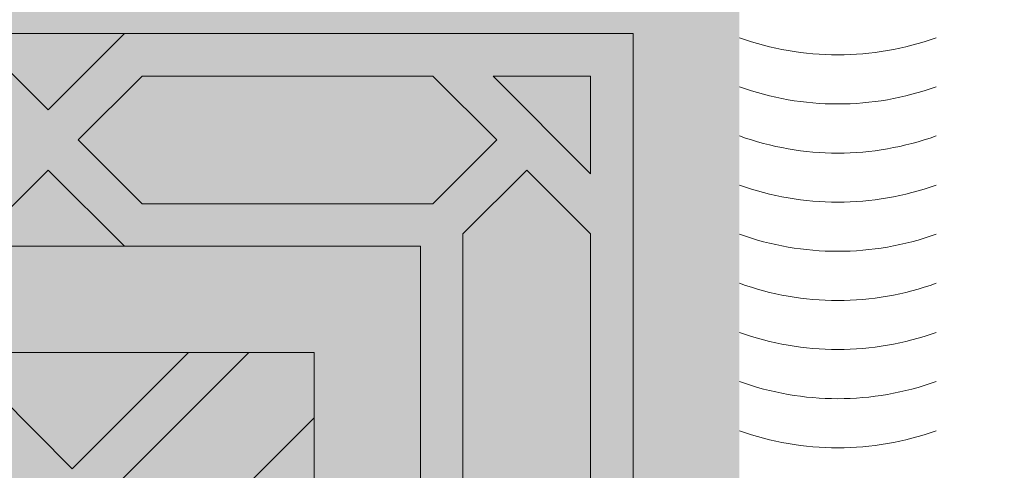
# Model space of a CAD drawing. Units: inches. Extents: x 844 to 2234, y 346 to 1084.
# Tile 86 of 93: x 2006.557 to 2012.46, y 710.224 to 712.926. Entities that reach past the tile are written whole.
import ezdxf

# ---------------------------------------------------------------- set-up
doc = ezdxf.new("R2010")
doc.units = ezdxf.units.IN
doc.header["$MEASUREMENT"] = 0
for name, color, linetype, lineweight in [('A-ANNO-DIMS', 2, 'Continuous', 18), ('furniture', 8, 'Continuous', 18), ('RA-AP-01$0$INT', 35, 'Continuous', 5)]:
    doc.layers.add(name, color=color, linetype=linetype, lineweight=lineweight)
doc.layers.add('RA-AP-01$0$FURN', color=3, linetype='Continuous')
doc.styles.get("Standard").update_dxf_attribs({"font": 'arial.ttf'})
doc.dimstyles.get("Standard").update_dxf_attribs({"dimtxt": 6, "dimasz": 3, "dimexe": 0.18, "dimexo": 0.0625, "dimgap": 0.09, "dimtad": 0, "dimtih": 1, "dimtoh": 1, "dimdec": 1, "dimzin": 0, "dimdsep": 46, "dimlunit": 3, "dimtxsty": 'Standard', "dimblk": 'ARCHTICK', "dimcen": 0.09, "dimadec": 0, "dimazin": 0, "dimtfac": 1, "dimtdec": 1, "dimtofl": 0, "dimtmove": 0, "dimatfit": 3, "dimfxl": 1, "dimtolj": 1, "dimtzin": 0, "dimarcsym": 0})

# ---------------------------------------------------------------- blocks, each defined once
blk = doc.blocks.new('A$C18D01794')
at = {"layer": 'RA-AP-01$0$INT'}
h = blk.add_hatch(color=256, dxfattribs=at)
h.paths.add_polyline_path([(4.355206456958071, -6.156712009588037), (4.355206456958071, -8.056712009588038), (5.455206456958072, -8.056712009588038), (5.455206456958072, -6.156712009588037)])
h.paths.add_polyline_path([(4.405206456958072, -8.006712009588039), (4.405206456958072, -6.206712009588038), (5.405206456958072, -6.206712009588038), (5.405206456958072, -8.006712009588039)], flags=16)
h = blk.add_hatch(color=256, dxfattribs=at)
h.paths.add_polyline_path([(4.505206456958071, -7.585498806127123), (4.46934859260189, -7.549640941759413), (4.505206456958071, -7.513783077414768), (4.505206456958071, -7.381963272220687), (4.469348592616735, -7.346105407867824), (4.505206456958071, -7.310247543514964), (4.505206456958071, -7.178427738324996), (4.469348592586679, -7.142569873965138), (4.505206456952245, -7.106712009588038), (4.476922185709333, -7.106712009588038), (4.455206456960671, -7.128427738343681), (4.433490728198047, -7.106712009588038), (4.405206456946033, -7.106712009588036), (4.441064321339216, -7.142569873969684), (4.40520645695807, -7.178427738362358), (4.405206456958072, -7.310247543472698), (4.441064321364728, -7.346105407867826), (4.40520645695807, -7.381963272262947), (4.40520645695807, -7.513783077378263), (4.441064321354429, -7.549640941786153), (4.405206456958072, -7.585498806170974), (4.405206456958072, -7.717318611286652), (4.441064321333084, -7.753176475673194), (4.405206456958072, -7.789034340036673), (4.405206456958072, -8.006712009588039), (4.644348592588106, -8.006712009588039), (4.680206456964639, -7.970854145211967), (4.716064321341165, -8.006712009588039), (4.869348592586113, -8.006712009588039), (4.905206456964143, -7.970854145210465), (4.941064321342174, -8.006712009588039), (5.094348592587118, -8.006712009588037), (5.130206456963649, -7.970854145211967), (5.166064321340178, -8.006712009588039), (5.405206456958072, -8.006712009588039), (5.405206456958072, -7.789034340024526), (5.369348592595202, -7.753176475673196), (5.40520645695807, -7.717318611298797), (5.40520645695807, -7.585498806158829), (5.369348592573859, -7.549640941786151), (5.40520645695807, -7.51378307739041), (5.40520645695807, -7.381963272250803), (5.36934859256356, -7.346105407867824), (5.405206456958072, -7.310247543484846), (5.405206456958072, -7.178427738350217), (5.369348592589068, -7.142569873969682), (5.405206456982249, -7.106712009588038), (5.376922185730244, -7.106712009588038), (5.355206456967613, -7.128427738343679), (5.333490728218955, -7.10671200958804), (5.305206456976043, -7.106712009588042), (5.341064321341609, -7.142569873965136), (5.305206456958072, -7.178427738337141), (5.305206456958072, -7.310247543502816), (5.34106432131155, -7.346105407867824), (5.305206456958072, -7.381963272232832), (5.30520645695807, -7.513783077402624), (5.341064321326395, -7.549640941759413), (5.305206456958072, -7.585498806139263), (5.305206456958072, -7.717318611299605), (5.341064321347738, -7.753176475677737), (5.305206456958072, -7.78903434007894), (5.30520645695807, -7.906712009588039), (5.166064321336834, -7.906712009588039), (5.130206456963647, -7.942569873961684), (5.094348592590464, -7.906712009588039), (4.941064321338827, -7.906712009588041), (4.905206456964145, -7.942569873963183), (4.869348592589459, -7.906712009588039), (4.716064321337822, -7.906712009588041), (4.680206456964641, -7.942569873961684), (4.644348592591453, -7.906712009588039), (4.505206456958071, -7.906712009588039), (4.505206456958071, -7.789034340066795), (4.469348592580545, -7.753176475677738), (4.505206456958071, -7.717318611311748)])
h.paths.add_polyline_path([(4.485206456974132, -7.709034340046354), (4.45520645695909, -7.739034340051736), (4.425206456974128, -7.709034340057131), (4.425206456993394, -7.593783077384998), (4.45520645699153, -7.563783077396511), (4.485206456993396, -7.593783077408017)], flags=16)
h.paths.add_polyline_path([(4.455206456954537, -7.767318611299197), (4.485206456958242, -7.797318611312542), (4.48520645695951, -7.912569873958716), (4.45520645695415, -7.942569873954422), (4.425206456957888, -7.912569873967813), (4.425206456957888, -7.797318611286197)], flags=16)
h.paths.add_polyline_path([(4.455206456964794, -7.535498806149051), (4.42520645696469, -7.5054988061393), (4.425206456983954, -7.390247543486406), (4.455206456990734, -7.360247543489279), (4.485206456983953, -7.39024754349214), (4.485206456964687, -7.505498806158811)], flags=16)
h.paths.add_polyline_path([(4.499348592588947, -7.926712009585049), (4.636064321340932, -7.926712009585049), (4.666064321342317, -7.956712009586821), (4.636064321343707, -7.986712009585048), (4.499348592575121, -7.986712009585048), (4.469348592591685, -7.956712009591957)], flags=16)
h.paths.add_polyline_path([(4.425206456957888, -7.940854145195974), (4.471064321332215, -7.986712009585049), (4.425206456957888, -7.986712009585049)], flags=16)
h.paths.add_polyline_path([(4.455206456990734, -7.331963272246367), (4.425206456989053, -7.301963272254337), (4.425206456969784, -7.186712009596224), (4.455206456965226, -7.156712009591144), (4.485206456969787, -7.186712009586051), (4.485206456989053, -7.301963272238404)], flags=16)
h.paths.add_polyline_path([(4.72434859258714, -7.926712009586255), (4.861064321340141, -7.926712009586248), (4.891064321340324, -7.956712009586823), (4.861064321340513, -7.986712009586252), (4.724348592586768, -7.986712009586252), (4.694348592586956, -7.956712009586821)], flags=16)
h.paths.add_polyline_path([(4.919348592587961, -7.956712009586821), (4.949348592588145, -7.92671200958625), (5.08606432134115, -7.926712009586253), (5.116064321341327, -7.956712009586823), (5.086064321341519, -7.986712009586252), (4.949348592587774, -7.986712009586252)], flags=16)
h.paths.add_polyline_path([(5.144348592585967, -7.956712009586823), (5.174348592587358, -7.926712009585049), (5.311064321339338, -7.926712009585049), (5.3410643213366, -7.956712009591957), (5.311064321353163, -7.986712009585048), (5.174348592584576, -7.986712009585048)], flags=16)
h.paths.add_polyline_path([(5.32520645693489, -7.593783077408021), (5.355206456936755, -7.563783077396511), (5.385206456934894, -7.593783077384998), (5.38520645695416, -7.709034340057128), (5.355206456969194, -7.739034340051736), (5.325206456954153, -7.709034340046352)], flags=16)
h.paths.add_polyline_path([(5.325206456970042, -7.797318611312542), (5.355206456973747, -7.767318611299197), (5.385206456970398, -7.7973186112862), (5.385206456970398, -7.912569873967816), (5.355206456974136, -7.942569873954422), (5.325206456968778, -7.912569873958716)], flags=16)
h.paths.add_polyline_path([(5.325206456963599, -7.505498806158811), (5.325206456944333, -7.39024754349214), (5.355206456937552, -7.360247543489279), (5.385206456944332, -7.39024754348641), (5.385206456963596, -7.505498806139303), (5.355206456963492, -7.53549880614905)], flags=16)
h.paths.add_polyline_path([(5.32520645693923, -7.301963272238403), (5.3252064569585, -7.186712009586051), (5.355206456963062, -7.156712009591142), (5.3852064569585, -7.186712009596224), (5.385206456939234, -7.301963272254338), (5.355206456937552, -7.331963272246369)], flags=16)
h.paths.add_polyline_path([(5.339348592596071, -7.986712009585048), (5.385206456970398, -7.940854145195972), (5.385206456970396, -7.986712009585048)], flags=16)
h = blk.add_hatch(color=256, dxfattribs=at)
h.paths.add_polyline_path([(4.469348592586677, -7.142569873965136), (4.505206456958073, -7.178427738324996), (4.505206456958071, -7.106712009582215)])
h.paths.add_polyline_path([(4.455206456960671, -7.128427738343681), (4.476922185709333, -7.106712009588038), (4.433490728198045, -7.106712009588038)])
h.paths.add_polyline_path([(4.405206456958073, -7.178427738362358), (4.441064321339218, -7.142569873969684), (4.40520645695807, -7.106712009600073)])
h.paths.add_polyline_path([(4.425206456989053, -7.301963272254335), (4.455206456990736, -7.331963272246371), (4.485206456989055, -7.301963272238399), (4.48520645696979, -7.186712009586054), (4.455206456965227, -7.15671200959114), (4.425206456969784, -7.186712009596224)])
h.paths.add_polyline_path([(4.505206456958073, -7.381963272220689), (4.505206456958071, -7.310247543514961), (4.469348592616738, -7.346105407867826)])
h.paths.add_polyline_path([(4.425206456964688, -7.5054988061393), (4.455206456964794, -7.535498806149051), (4.485206456964689, -7.505498806158811), (4.485206456983951, -7.390247543492138), (4.455206456990736, -7.360247543489277), (4.425206456983956, -7.39024754348641)])
h.paths.add_polyline_path([(4.425206456974126, -7.709034340057128), (4.455206456959092, -7.739034340051736), (4.485206456974132, -7.709034340046356), (4.485206456993396, -7.593783077408017), (4.45520645699153, -7.563783077396511), (4.425206456993394, -7.593783077384999)])
h.paths.add_polyline_path([(4.46934859260189, -7.549640941759415), (4.505206456958071, -7.585498806127123), (4.505206456958073, -7.513783077414766)])
h.paths.add_polyline_path([(4.405206456958073, -7.585498806170972), (4.441064321354427, -7.549640941786151), (4.405206456958072, -7.513783077378263)])
h.paths.add_polyline_path([(4.405206456958072, -7.789034340036673), (4.441064321333084, -7.753176475673194), (4.405206456958072, -7.71731861128665)])
h.paths.add_polyline_path([(4.469348592580547, -7.75317647567774), (4.505206456958071, -7.789034340066795), (4.505206456958071, -7.717318611311744)])
h.paths.add_polyline_path([(4.425206456957888, -7.912569873967814), (4.45520645695415, -7.942569873954422), (4.485206456959507, -7.912569873958718), (4.48520645695824, -7.797318611312542), (4.455206456954537, -7.767318611299197), (4.425206456957888, -7.797318611286202)])
h.paths.add_polyline_path([(4.425206456957888, -7.986712009585049), (4.471064321332215, -7.986712009585049), (4.425206456957888, -7.940854145195972)])
h.paths.add_polyline_path([(4.499348592575121, -7.986712009585048), (4.636064321343707, -7.986712009585049), (4.666064321342317, -7.956712009586823), (4.636064321340932, -7.926712009585049), (4.499348592588945, -7.926712009585049), (4.469348592591685, -7.95671200959196)])
h.paths.add_polyline_path([(4.680206456964641, -7.942569873961684), (4.716064321337824, -7.906712009588039), (4.644348592591454, -7.906712009588039)])
h.paths.add_polyline_path([(4.644348592588108, -8.006712009588039), (4.716064321341167, -8.006712009588039), (4.680206456964637, -7.970854145211964)])
h.paths.add_polyline_path([(4.724348592586768, -7.98671200958625), (4.861064321340514, -7.986712009586252), (4.891064321340324, -7.956712009586819), (4.861064321340141, -7.92671200958625), (4.724348592587134, -7.926712009586255), (4.694348592586957, -7.956712009586821)])
h.paths.add_polyline_path([(4.905206456964143, -7.942569873963183), (4.941064321338827, -7.906712009588039), (4.869348592589457, -7.906712009588037)])
h.paths.add_polyline_path([(4.869348592586113, -8.006712009588039), (4.941064321342172, -8.006712009588037), (4.905206456964145, -7.970854145210463)])
h.paths.add_polyline_path([(4.949348592587774, -7.986712009586252), (5.086064321341521, -7.986712009586252), (5.116064321341329, -7.956712009586823), (5.08606432134115, -7.926712009586253), (4.949348592588145, -7.92671200958625), (4.919348592587961, -7.956712009586819)])
h.paths.add_polyline_path([(5.130206456963645, -7.942569873961684), (5.166064321336834, -7.906712009588039), (5.094348592590464, -7.906712009588039)])
h.paths.add_polyline_path([(5.094348592587119, -8.006712009588039), (5.166064321340178, -8.006712009588039), (5.130206456963651, -7.970854145211967)])
h.paths.add_polyline_path([(5.174348592584578, -7.986712009585048), (5.311064321353163, -7.986712009585048), (5.341064321336602, -7.956712009591958), (5.31106432133934, -7.926712009585049), (5.174348592587352, -7.926712009585049), (5.144348592585969, -7.956712009586823)])
h.paths.add_polyline_path([(5.325206456968778, -7.912569873958718), (5.355206456974136, -7.942569873954422), (5.385206456970396, -7.912569873967814), (5.385206456970396, -7.797318611286199), (5.355206456973747, -7.767318611299197), (5.325206456970044, -7.797318611312544)])
h.paths.add_polyline_path([(5.339348592596073, -7.986712009585048), (5.385206456970396, -7.986712009585049), (5.385206456970398, -7.94085414519597)])
h.paths.add_polyline_path([(5.325206456954155, -7.709034340046354), (5.355206456969194, -7.739034340051734), (5.38520645695416, -7.709034340057128), (5.385206456934896, -7.593783077384999), (5.355206456936758, -7.563783077396513), (5.325206456934888, -7.593783077408019)])
h.paths.add_polyline_path([(5.305206456958072, -7.789034340078938), (5.341064321347739, -7.753176475677738), (5.305206456958072, -7.717318611299605)])
h.paths.add_polyline_path([(5.369348592595204, -7.753176475673194), (5.40520645695807, -7.789034340024526), (5.405206456958072, -7.717318611298798)])
h.paths.add_polyline_path([(5.405206456958072, -7.585498806158831), (5.405206456958072, -7.513783077390407), (5.369348592573857, -7.549640941786151)])
h.paths.add_polyline_path([(5.305206456958072, -7.585498806139266), (5.341064321326393, -7.549640941759413), (5.305206456958072, -7.513783077402626)])
h.paths.add_polyline_path([(5.325206456963599, -7.50549880615881), (5.355206456963494, -7.535498806149055), (5.385206456963598, -7.505498806139302), (5.385206456944334, -7.390247543486411), (5.355206456937552, -7.360247543489279), (5.325206456944333, -7.39024754349214)])
h.paths.add_polyline_path([(5.305206456958072, -7.38196327223283), (5.341064321311551, -7.346105407867824), (5.305206456958072, -7.31024754350282)])
h.paths.add_polyline_path([(5.325206456939231, -7.301963272238404), (5.355206456937552, -7.331963272246369), (5.385206456939235, -7.301963272254335), (5.385206456958502, -7.186712009596224), (5.355206456963061, -7.156712009591142), (5.3252064569585, -7.186712009586051)])
h.paths.add_polyline_path([(5.404581768715993, -7.381338584008926, -0.001217816984214), (5.405206456958072, -7.381112009582329), (5.405206456958072, -7.310247543484846), (5.369348592563558, -7.346105407867826)])
h.paths.add_polyline_path([(5.36934859258907, -7.142569873969684), (5.40520645695807, -7.178427738350215), (5.405206456958072, -7.106712009612218)])
h.paths.add_polyline_path([(5.355206456967613, -7.128427738343683), (5.376922185730239, -7.106712009588038), (5.333490728218953, -7.10671200958804)])
h.paths.add_polyline_path([(5.30520645695807, -7.178427738337139), (5.341064321341609, -7.142569873965134), (5.305206456958074, -7.10671200957007)])
blk.add_hatch(color=256, dxfattribs=at).paths.add_polyline_path([(4.505206456958071, -7.906712009588039), (5.305206456958072, -7.906712009588039), (5.305206456958072, -7.106712009588038), (5.255206456951893, -7.106712009588036), (5.25520645694868, -7.856712009570104), (4.555206456959269, -7.856712009588616), (4.555206456956052, -7.106712009588038), (4.505206456958073, -7.106712009588038)])
h = blk.add_hatch(color=256, dxfattribs=at)
h.paths.add_polyline_path([(4.585917135068448, -7.856712009587804), (4.614201406330596, -7.856712009587056), (4.668846067270487, -7.802067348644738), (4.723490728212344, -7.856712009584164), (4.771774999457151, -7.856712009582887), (4.826419660396886, -7.80206734864072), (4.862780050090322, -7.838427738332541), (4.844495778842715, -7.856712009580965), (4.862780050090411, -7.856712009580482), (4.905206456960182, -7.814285602707865), (4.947632863832445, -7.856712009578238), (4.965917135079675, -7.856712009577755), (4.947632863831759, -7.838427738330656), (4.983993253523576, -7.802067348637219), (5.038637914464627, -7.856712009575829), (5.08692218571208, -7.856712009574554), (5.141566846649976, -7.802067348634224), (5.196211507589851, -7.856712009571666), (5.224495778822615, -7.856712009570916), (4.905206456953975, -7.537422687702283)])
h.paths.add_polyline_path([(4.895206456956031, -7.575706958950402), (4.895206456958921, -7.684996280828174), (4.840561796018589, -7.630351619890275)], flags=16)
h.paths.add_polyline_path([(4.915206456955638, -7.575706958949956), (4.969851117895509, -7.630351619887399), (4.915206456957609, -7.684996280827732)], flags=16)
h.paths.add_polyline_path([(4.826419660395175, -7.644493755514321), (4.881064321335613, -7.699138416452331), (4.771774999456703, -7.69913841645522)], flags=16)
h.paths.add_polyline_path([(4.983993253519558, -7.644493755510815), (5.038637914460456, -7.699138416449285), (4.929348592581548, -7.69913841645126)], flags=16)
h.paths.add_polyline_path([(4.881064321336025, -7.719138416452334), (4.826419660397532, -7.773783077393256), (4.771774999457062, -7.719138416455217)], flags=16)
h.paths.add_polyline_path([(4.929348592582019, -7.71913841645126), (5.038637914460982, -7.719138416449284), (4.983993253522945, -7.773783077389749)], flags=16)
h.paths.add_polyline_path([(4.895206456960191, -7.733280552075633), (4.895206456962115, -7.806001331460164), (4.876922185715016, -7.824285602708492), (4.840561796021581, -7.787925213016675)], flags=16)
h.paths.add_polyline_path([(4.915206456958487, -7.733280552075187), (4.969851117899527, -7.787925213013798), (4.933490728206909, -7.824285602708034), (4.9152064569598, -7.806001331461736)], flags=16)
h.paths.add_polyline_path([(4.757632863832376, -7.733280552079264), (4.812277524772842, -7.787925213017304), (4.757632863834348, -7.842569873958233)], flags=16)
h.paths.add_polyline_path([(4.737632863832376, -7.73328055207979), (4.737632863834348, -7.842569873958701), (4.682988202893906, -7.787925213020692)], flags=16)
h.paths.add_polyline_path([(5.05278005008503, -7.733280552072701), (5.052780050087917, -7.842569873951664), (4.998135389146995, -7.787925213013169)], flags=16)
h.paths.add_polyline_path([(5.072780050085024, -7.733280552072333), (5.127424711025931, -7.787925213010806), (5.072780050087916, -7.842569873951244)], flags=16)
h.paths.add_polyline_path([(4.935917135072783, -7.506712009583784), (5.255206456948811, -7.826001331459767), (5.255206456948932, -7.797717060211899), (5.200561796010279, -7.743072399273238), (5.255206456949403, -7.688427738334128), (5.25520645694961, -7.640143467086677), (5.200561796009787, -7.585498806146837), (5.236922185702417, -7.549138416454212), (5.255206456949919, -7.56742268770172), (5.255206456949998, -7.549138416454178), (5.212780050078687, -7.506712009583814), (5.25520645695036, -7.464285602712145), (5.255206456950438, -7.446001331464763), (5.236922185702424, -7.464285602712779), (5.200561796009796, -7.427925213020149), (5.255206456950753, -7.373280552079203), (5.25520645695096, -7.324996280834394), (5.200561796010322, -7.270351619893748), (5.255206456951428, -7.215706958952649), (5.255206456951547, -7.187422687705071)])
h.paths.add_polyline_path([(5.042988202883395, -7.42792521302065), (5.097632863823085, -7.373280552080975), (5.097632863822622, -7.482569873959883)], flags=16)
h.paths.add_polyline_path([(5.028846067259663, -7.442067348644384), (5.083490728198774, -7.496712009583504), (4.974201406321001, -7.496712009583035)], flags=16)
h.paths.add_polyline_path([(5.117632863823087, -7.37328055208089), (5.172277524762331, -7.42792521302015), (5.11763286382262, -7.482569873959851)], flags=16)
h.paths.add_polyline_path([(5.08349072819877, -7.516712009582191), (5.028846067259652, -7.571356670521302), (4.974201406320998, -7.516712009582638)], flags=16)
h.paths.add_polyline_path([(5.131774999446817, -7.35913841645716), (5.186419660386065, -7.413783077396415), (5.241064321325782, -7.359138416456712)], flags=17)
h.paths.add_polyline_path([(5.131774999446228, -7.496712009583703), (5.186419660386065, -7.442067348643883), (5.222780050079488, -7.478427738337313), (5.204495778832781, -7.496712009584014)], flags=16)
h.paths.add_polyline_path([(5.097632863822613, -7.530854145205813), (5.097632863823061, -7.640143467084723), (5.042988202883383, -7.585498806145032)], flags=16)
h.paths.add_polyline_path([(5.131774999446899, -7.339138416457162), (5.241064321325809, -7.339138416456712), (5.186419660386591, -7.284493755517479)], flags=17)
h.paths.add_polyline_path([(5.131774999446226, -7.516712009581999), (5.204495778830767, -7.516712009581702), (5.22278005007868, -7.534996280829206), (5.186419660386049, -7.571356670521828)], flags=16)
h.paths.add_polyline_path([(5.11763286382262, -7.530854145205852), (5.17227752476232, -7.585498806145562), (5.117632863823064, -7.64014346708481)], flags=16)
h.paths.add_polyline_path([(5.186419660386069, -7.599640941770585), (5.241064321325754, -7.654285602710281), (5.131774999446791, -7.654285602709814)], flags=16)
h.paths.add_polyline_path([(5.131774999446872, -7.674285602709813), (5.24106432132578, -7.674285602710282), (5.186419660386554, -7.728930263649504)], flags=16)
h.paths.add_polyline_path([(5.255206456951811, -7.126001331467467), (5.255206456951895, -7.106712009588038), (4.555206456956052, -7.106712009588038), (4.555206456956136, -7.12600133146746), (4.905206456953973, -7.476001331465289)])
h.paths.add_polyline_path([(4.983993253513404, -7.368930263651977), (4.92934859257295, -7.314285602713969), (5.03863791445186, -7.314285602711063)], flags=16)
h.paths.add_polyline_path([(4.969851117889988, -7.383072399276016), (4.915206456952556, -7.437717060215906), (4.915206456949648, -7.328427738338133)], flags=16)
h.paths.add_polyline_path([(4.929348592572535, -7.294285602713971), (4.983993253511019, -7.239640941773039), (5.038637914451496, -7.294285602711065)], flags=16)
h.paths.add_polyline_path([(5.052780050074912, -7.280143467087016), (4.998135389134438, -7.225498806148989), (5.052780050072919, -7.170854145208052)], flags=16)
h.paths.add_polyline_path([(5.07278005007491, -7.280143467086489), (5.072780050072918, -7.170854145207579), (5.127424711013374, -7.225498806145578)], flags=16)
h.paths.add_polyline_path([(4.89520645695295, -7.437717060216355), (4.840561796013067, -7.383072399278919), (4.895206456950961, -7.328427738338582)], flags=16)
h.paths.add_polyline_path([(4.915206456948365, -7.280143467090674), (4.915206456946434, -7.207422687704125), (4.933490728192729, -7.18913841645701), (4.969851117886972, -7.225498806149623)], flags=16)
h.paths.add_polyline_path([(4.881064321327021, -7.314285602715054), (4.82641966038902, -7.368930263655506), (4.771774999448108, -7.314285602717047)], flags=16)
h.paths.add_polyline_path([(4.895206456950073, -7.280143467091125), (4.840561796009022, -7.225498806152518), (4.876922185700835, -7.18913841645908), (4.895206456948749, -7.207422687706589)], flags=16)
h.paths.add_polyline_path([(4.983993253510392, -7.211356670525576), (4.947632863816944, -7.174996280833758), (4.965917135064043, -7.156712009585847), (5.038637914448995, -7.156712009584522)], flags=16)
h.paths.add_polyline_path([(4.881064321326543, -7.294285602715056), (4.771774999447578, -7.294285602717046), (4.826419660385607, -7.239640941776569)], flags=16)
h.paths.add_polyline_path([(4.905206456946447, -7.19913841645844), (4.862780050074785, -7.156712009587725), (4.947632863816685, -7.156712009586302)], flags=16)
h.paths.add_polyline_path([(5.14156684663679, -7.211356670521528), (5.086922185696452, -7.156712009583639), (5.196211507574223, -7.156712009581651)], flags=16)
h.paths.add_polyline_path([(4.8264196603837, -7.211356670529104), (4.771774999442643, -7.156712009590501), (4.8444957788276, -7.156712009588568), (4.862780050075511, -7.17499628083566)], flags=16)
h.paths.add_polyline_path([(4.812277524760289, -7.225498806153156), (4.757632863822258, -7.28014346709363), (4.757632863819352, -7.170854145214669)], flags=16)
h.paths.add_polyline_path([(4.73763286382226, -7.280143467093997), (4.682988202881349, -7.22549880615554), (4.737632863819352, -7.170854145215086)], flags=16)
h.paths.add_polyline_path([(4.723490728195188, -7.156712009591787), (4.668846067257299, -7.211356670532127), (4.614201406317417, -7.156712009594693)], flags=16)
h.paths.add_polyline_path([(4.597632863829262, -7.506712009583814), (4.555206456957951, -7.54913841645418), (4.555206456958029, -7.56742268770172), (4.573490728205535, -7.549138416454212), (4.609851117898167, -7.585498806146839), (4.555206456958338, -7.640143467086675), (4.555206456958546, -7.688427738334125), (4.60985111789767, -7.743072399273238), (4.555206456959015, -7.797717060211899), (4.555206456959138, -7.826001331459767), (4.874495778835167, -7.506712009583786), (4.5552064569564, -7.187422687705062), (4.555206456956523, -7.215706958952644), (4.609851117897629, -7.270351619893746), (4.555206456956988, -7.324996280834396), (4.555206456957198, -7.373280552079195), (4.609851117898153, -7.427925213020147), (4.573490728205528, -7.464285602712779), (4.555206456957507, -7.446001331464756), (4.555206456957585, -7.464285602712143)])
h.paths.add_polyline_path([(4.712780050085332, -7.482569873959882), (4.712780050084863, -7.373280552080972), (4.767424711024555, -7.42792521302065)], flags=16)
h.paths.add_polyline_path([(4.726922185709173, -7.496712009583504), (4.781566846648288, -7.442067348644384), (4.836211507586949, -7.496712009583033)], flags=16)
h.paths.add_polyline_path([(4.692780050085327, -7.482569873959851), (4.638135389145619, -7.427925213020149), (4.692780050084865, -7.373280552080892)], flags=16)
h.paths.add_polyline_path([(4.726922185709182, -7.516712009582191), (4.836211507586949, -7.51671200958264), (4.7815668466483, -7.571356670521304)], flags=16)
h.paths.add_polyline_path([(4.678637914461726, -7.496712009583706), (4.605917135075169, -7.496712009584014), (4.587632863828464, -7.478427738337311), (4.623993253521887, -7.442067348643881)], flags=16)
h.paths.add_polyline_path([(4.712780050085336, -7.530854145205816), (4.767424711024568, -7.585498806145034), (4.71278005008489, -7.640143467084724)], flags=16)
h.paths.add_polyline_path([(4.678637914461726, -7.516712009582001), (4.623993253521899, -7.571356670521829), (4.587632863829271, -7.534996280829206), (4.605917135077185, -7.5167120095817)], flags=16)
h.paths.add_polyline_path([(4.692780050085336, -7.530854145205848), (4.692780050084889, -7.64014346708481), (4.638135389145632, -7.585498806145562)], flags=16)
h.paths.add_polyline_path([(4.623993253521885, -7.413783077396415), (4.678637914461131, -7.359138416457161), (4.56934859258217, -7.359138416456712)], flags=17)
h.paths.add_polyline_path([(4.623993253521901, -7.599640941770568), (4.678637914461158, -7.654285602709814), (4.569348592582195, -7.654285602710281)], flags=16)
h.paths.add_polyline_path([(4.678637914461051, -7.339138416457162), (4.623993253521361, -7.284493755517479), (4.569348592582143, -7.339138416456712)], flags=17)
h.paths.add_polyline_path([(4.678637914461076, -7.674285602709813), (4.623993253521399, -7.728930263649504), (4.569348592582167, -7.674285602710281)], flags=16)
h = blk.add_hatch(color=256, dxfattribs=at)
h.paths.add_polyline_path([(4.905206456954232, -7.537422687702028), (4.874495778835232, -7.506712009583718), (4.555206456959138, -7.826001331459766), (4.555206456959269, -7.856712009588616), (4.585917135068449, -7.856712009587804)])
h.paths.add_polyline_path([(4.935917135072152, -7.506712009583152), (4.905206456953497, -7.537422687701806), (5.224495778822614, -7.856712009570917), (5.255206456948681, -7.856712009570104), (5.255206456948813, -7.826001331459768)])
h.paths.add_polyline_path([(5.255206456951549, -7.18742268770507), (5.255206456951813, -7.126001331467461), (4.905206456953563, -7.476001331465701), (4.935917135072559, -7.506712009584006)])
h.paths.add_polyline_path([(4.874495778835167, -7.506712009583785), (4.905206456953818, -7.476001331465132), (4.555206456956135, -7.126001331467458), (4.555206456956399, -7.187422687705064)])
h = blk.add_hatch(color=256, dxfattribs=at)
h.paths.add_polyline_path([(4.969851117891331, -7.630351619889621), (4.915206456952669, -7.575706958950966), (4.915206456952222, -7.684996280828739)])
h.paths.add_polyline_path([(4.895206456953064, -7.575706958950968), (4.840561796014413, -7.630351619889628), (4.895206456953533, -7.684996280828741)])
h.paths.add_polyline_path([(4.826419660390684, -7.644493755513362), (4.771774999451003, -7.699138416453052), (4.881064321329913, -7.699138416452587)])
h.paths.add_polyline_path([(4.881064321329884, -7.719138416452585), (4.771774999450921, -7.719138416453052), (4.82641966039018, -7.773783077392298)])
h.paths.add_polyline_path([(4.895206456953734, -7.733280552076196), (4.840561796013912, -7.787925213016031), (4.876922185707337, -7.824285602709455), (4.895206456954043, -7.806001331462747)])
h.paths.add_polyline_path([(4.862780050082808, -7.838427738332388), (4.826419660390178, -7.802067348639763), (4.771774999450351, -7.856712009579595), (4.844495778835303, -7.856712009579895)])
h.paths.add_polyline_path([(4.812277524766446, -7.787925213016036), (4.757632863827191, -7.733280552076788), (4.757632863826741, -7.842569873955747)])
h.paths.add_polyline_path([(4.737632863827191, -7.733280552076863), (4.682988202887508, -7.787925213016558), (4.737632863826743, -7.842569873955778)])
h.paths.add_polyline_path([(4.668846067263777, -7.802067348640287), (4.614201406325123, -7.856712009578949), (4.723490728202894, -7.856712009579402)])
h.paths.add_polyline_path([(4.905206456953846, -7.814285602708654), (4.862780050082654, -7.856712009579847), (4.947632863824561, -7.85671200958032)])
h.paths.add_polyline_path([(4.915206456952028, -7.733280552076195), (4.91520645695173, -7.806001331460731), (4.933490728199234, -7.824285602708648), (4.96985111789186, -7.787925213016022)])
h.paths.add_polyline_path([(5.038637914454841, -7.719138416453029), (4.929348592575874, -7.71913841645258), (4.983993253515593, -7.773783077392289)])
h.paths.add_polyline_path([(4.983993253515065, -7.644493755513352), (4.929348592575849, -7.699138416452582), (5.038637914454755, -7.699138416453031)])
h.paths.add_polyline_path([(5.052780050079843, -7.73328055207676), (4.998135389140595, -7.787925213016018), (5.052780050080309, -7.842569873955721)])
h.paths.add_polyline_path([(4.983993253516868, -7.802067348639752), (4.947632863824241, -7.838427738332383), (4.965917135071747, -7.856712009579888), (5.038637914456701, -7.856712009579572)])
h.paths.add_polyline_path([(5.127424711019533, -7.787925213016519), (5.072780050079843, -7.733280552076838), (5.07278005008031, -7.842569873955751)])
h.paths.add_polyline_path([(5.141566846643269, -7.802067348640248), (5.086922185704154, -7.85671200957937), (5.196211507581929, -7.856712009578901)])
for p, q in [((4.555206456956052, -7.106712009588036), (4.555206456959269, -7.856712009588616)), ((4.874495778835167, -7.506712009583786), (4.555206456959136, -7.826001331459769)), ((4.905206456953975, -7.537422687702283), (4.585917135071132, -7.856712009585121)), ((4.425206456957888, -7.797318611286199), (4.425206456957888, -7.912569873967814)), ((4.485206456959509, -7.912569873958718), (4.485206456958242, -7.797318611312544)), ((4.614201406333045, -7.85671200958461), (4.668846067270487, -7.802067348644737)), ((4.723490728210815, -7.856712009582635), (4.668846067270487, -7.802067348644737)), ((4.555206456959269, -7.856712009588616), (5.255206456948681, -7.856712009570104)), ((5.267206456961765, -7.906712009586254), (4.543206456966523, -7.906712009586254)), ((5.2672064569642, -7.906712009586255), (4.54320645696085, -7.906712009586255)), ((4.644348592589667, -7.906712009586254), (4.680206456964639, -7.942569873961684)), ((4.716064321339607, -7.906712009586254), (4.680206456964639, -7.942569873961684)), ((4.425206456957888, -7.912569873967814), (4.45520645695415, -7.942569873954422)), ((4.485206456959509, -7.912569873958718), (4.45520645695415, -7.942569873954422)), ((4.499348592588947, -7.926712009585049), (4.469348592591685, -7.956712009591957)), ((4.636064321340932, -7.926712009585049), (4.499348592588947, -7.926712009585049)), ((4.636064321340932, -7.926712009585049), (4.666064321342317, -7.956712009586823)), ((4.425206456957888, -7.940854145195974), (4.425206456957888, -7.986712009585049)), ((4.471064321332213, -7.986712009585048), (4.425206456957888, -7.940854145195974)), ((4.499348592575123, -7.986712009585048), (4.469348592591685, -7.956712009591957)), ((4.636064321343709, -7.986712009585049), (4.666064321342317, -7.956712009586823)), ((4.644348592589893, -8.006712009586252), (4.680206456964637, -7.970854145211966)), ((4.716064321339382, -8.006712009586252), (4.680206456964637, -7.970854145211966)), ((4.471064321332213, -7.986712009585048), (4.425206456957888, -7.986712009585049)), ((4.636064321343709, -7.986712009585049), (4.499348592575123, -7.986712009585048))]:
    blk.add_line(p, q, dxfattribs=at)
for points in [[(5.405206456958072, -8.006712009588039), (4.405206456958072, -8.006712009588039), (4.405206456958072, -7.106712009588038)], [(5.305206456958072, -7.106712009588038), (5.305206456958072, -7.906712009588039), (4.505206456958071, -7.906712009588039), (4.505206456958071, -7.106712009588038)]]:
    blk.add_lwpolyline(points, dxfattribs=at)
for centre in [(4.309006456952313, -7.948364458284338), (4.309006456952086, -7.971464458286042), (4.30900645694913, -7.994564458281608), (4.309006456948902, -8.017664458286497), (4.309006456951858, -8.040764458285018), (4.309006456950267, -8.063864458283767), (4.309006456948448, -8.086964458285472), (4.309006456948448, -8.11006445828422), (4.309006456946856, -8.13316445828297)]:
    blk.add_arc(centre, 0.136414042854523, 70.20384312815696, 109.7961568705686, dxfattribs=at)
blk = doc.blocks.new('A$C5D2F253E')
at = {"layer": 'RA-AP-01$0$FURN', "xscale": -0.7999999999883585, "yscale": 0.7999999999883585, "zscale": 0.8, "rotation": 90}
blk.add_blockref('A$C18D01794', (-5.687757199772477, 4.75791982714071), dxfattribs=at)
blk = doc.blocks.new('_ArchTick')
at = {"color": 0, "linetype": 'ByBlock', "const_width": 0.15}
blk.add_lwpolyline([(-0.5, -0.5), (0.5, 0.5)], dxfattribs=at)
blk = doc.blocks.new('*D121')
at = {"layer": 'A-ANNO-DIMS', "color": 0, "lineweight": -2, "transparency": 16777216}
for p, q in [((2030.271987351997, 734.262611118704), (2040.245275089302, 734.262611118704)), ((2040.065275089302, 734.262611118704), (2040.065275089302, 704.6043509484256)), ((2040.065275089302, 668.557359536674), (2040.065275089302, 698.2156197069523)), ((2030.271987351997, 668.557359536674), (2040.245275089302, 668.557359536674))]:
    blk.add_line(p, q, dxfattribs=at)
at = {"layer": 'Defpoints', "color": 0, "transparency": 16777216}
for p in [(2030.209487351997, 734.262611118704), (2040.065275089302, 734.262611118704), (2030.209487351997, 668.557359536674)]:
    blk.add_point(p, dxfattribs=at)
at = {"layer": 'A-ANNO-DIMS', "color": 0, "lineweight": -2, "transparency": 16777216, "xscale": 3, "yscale": 3, "zscale": 3}
for p, rotation in [((2040.065275089302, 734.262611118704), 90), ((2040.065275089302, 668.557359536674), 270)]:
    blk.add_blockref('_ArchTick', p, dxfattribs=dict(at, rotation=rotation))
at = {"layer": 'A-ANNO-DIMS', "color": 0, "transparency": 16777216, "insert": (2040.065275089302, 701.4099853276883), "char_height": 6, "attachment_point": 5}
blk.add_mtext('\\A1;LOUNGE SET 5\'-5 1/2" TYP.', dxfattribs=at)

msp = doc.modelspace()

# ---------------------------------------------------------------- block references
at = {"layer": 'furniture', "xscale": -15.94108302203742, "yscale": 15.94108302203742, "zscale": 15.94108302203742, "rotation": 270}
msp.add_blockref('A$C5D2F253E', (1990.567271852805, 701.4028671565849), dxfattribs=at)

# ---------------------------------------------------------------- dimensions: what is measured, and where the dimension line sits
at = {"layer": 'A-ANNO-DIMS'}
dim = msp.add_linear_dim(base=(2040.065275089302, 734.262611118704), p1=(2030.209487351996, 668.5573595366737), p2=(2030.209487351996, 734.2626111187037), angle=90, text='LOUNGE SET <> TYP.', dimstyle='Standard', override={"dimdec": 1, "dimlfac": 1, "dimrnd": 0, "dimzin": 1, "dimdsep": 46, "dimlunit": 4, "dimfrac": 2}, dxfattribs=at)
dim.commit()
dim.dimension.update_dxf_attribs({"geometry": '*D121', "text_midpoint": (2040.065275089302, 701.4099853276883)})

doc.saveas('drawing.dxf')
